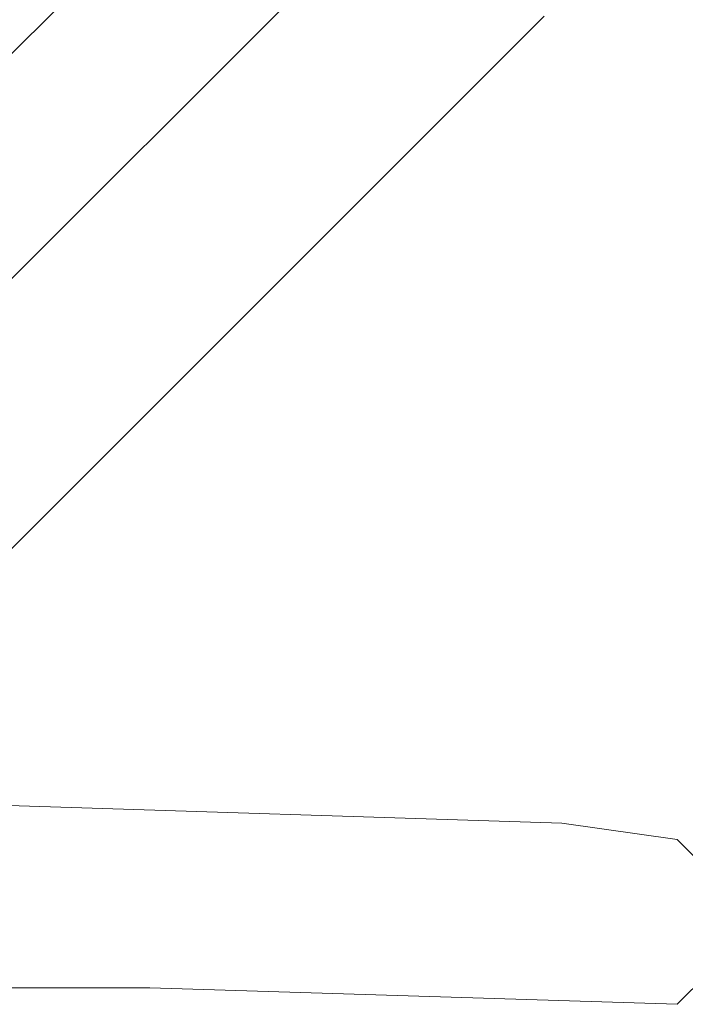
# Model space of a CAD drawing. Units: inches. Extents: x 375 to 1122, y 27 to 1069.
# Tile 39 of 155: x 715.392 to 717.878, y 296.625 to 300.305. Entities that reach past the tile are written whole.
import ezdxf

# ---------------------------------------------------------------- set-up
doc = ezdxf.new("R2010")
doc.units = ezdxf.units.IN
doc.layers.add('Furniture', color=30, linetype='Continuous', lineweight=18)

# ---------------------------------------------------------------- blocks, each defined once
blk = doc.blocks.new('A$C403C54AD')
at = {"invisible_edges": 5}
for points in [[(1.238741, 0.825561, -0.024899), (1.229506, 0.825561, -0.024899), (1.226428, 0.822483, -0.024899), (1.24182, 0.822483, -0.024899)], [(1.238741, 0.825561, -0.026438), (1.229506, 0.825561, -0.026438), (1.226428, 0.822483, -0.026438), (1.24182, 0.822483, -0.026438)], [(1.229506, 0.825561, -0.026438), (1.229506, 0.825561, -0.024899), (1.226428, 0.822483, -0.024899), (1.226428, 0.822483, -0.026438)], [(1.24182, 0.822483, -0.024899), (1.24182, 0.822483, -0.026438), (1.238741, 0.825561, -0.026438), (1.238741, 0.825561, -0.024899)], [(1.226428, 0.822483, -0.024899), (1.24182, 0.822483, -0.024899), (1.24028, 0.773228, -0.024899), (1.224889, 0.811708, -0.024899)], [(1.226428, 0.822483, -0.026438), (1.24182, 0.822483, -0.026438), (1.24028, 0.773228, -0.026438), (1.224889, 0.811708, -0.026438)], [(1.226428, 0.822483, -0.024899), (1.226428, 0.822483, -0.026438), (1.224889, 0.811708, -0.026438), (1.224889, 0.811708, -0.024899)], [(1.24028, 0.773228, -0.026438), (1.24028, 0.773228, -0.024899), (1.24182, 0.822483, -0.024899), (1.24182, 0.822483, -0.026438)], [(1.24028, 0.773228, -0.024899), (1.224889, 0.811708, -0.024899), (1.22181, 0.714739, -0.024899), (1.24028, 0.714739, -0.024899)], [(1.24028, 0.773228, -0.026438), (1.224889, 0.811708, -0.026438), (1.22181, 0.714739, -0.026438), (1.24028, 0.714739, -0.026438)], [(1.224889, 0.811708, -0.026438), (1.224889, 0.811708, -0.024899), (1.22181, 0.714739, -0.024899), (1.22181, 0.714739, -0.026438)], [(1.24028, 0.714739, -0.024899), (1.24028, 0.714739, -0.026438), (1.24028, 0.773228, -0.026438), (1.24028, 0.773228, -0.024899)]]:
    blk.add_3dface(points, dxfattribs=at)
at = {"linetype": 'ByBlock', "invisible_edges": 5}
for points in [[(1.170847, 0.742445, -0.02259), (1.200173, 0.759376, -0.013355), (1.149468, 0.81008, -0.013355), (1.132537, 0.780755, -0.02259)], [(1.200173, 0.759376, -0.008737), (1.184177, 0.750141, -0.008737), (1.140233, 0.794084, -0.008737), (1.149468, 0.81008, -0.008737)], [(1.184177, 0.750141, -0.008737), (1.168181, 0.740905, -0.014894), (1.130998, 0.778089, -0.014894), (1.140233, 0.794084, -0.008737)], [(1.162849, 0.737827, -0.031825), (1.170847, 0.742445, -0.02259), (1.132537, 0.780755, -0.02259), (1.12792, 0.772757, -0.031825)], [(1.168181, 0.740905, -0.014894), (1.080205, 0.690112, -0.014894), (1.080205, 0.690112, -0.014894), (1.130998, 0.778089, -0.014894)]]:
    blk.add_3dface(points, dxfattribs=at)
at = {"linetype": 'ByBlock'}
blk.add_3dface([(1.200173, 0.759376, -0.013355), (1.200173, 0.759376, -0.008737), (1.149468, 0.81008, -0.008737), (1.149468, 0.81008, -0.013355)], dxfattribs=at)

msp = doc.modelspace()

# ---------------------------------------------------------------- block references
at = {"layer": 'Furniture', "xscale": 39.9918517141215, "yscale": 39.9918517141215, "zscale": 39.9918517141215, "rotation": 270}
msp.add_blockref('A$C403C54AD', (684.9549, 346.2875, 0.024), dxfattribs=at)

doc.saveas('drawing.dxf')
